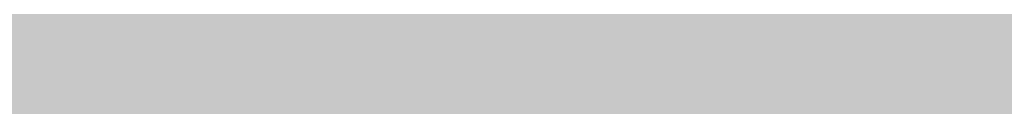
# Model space of a CAD drawing. Units: millimetres. Extents: x 0 to 2267, y 0 to 1823.
# Tile 53 of 256: x 1596.855 to 1600.369, y 1226.718 to 1227.02. Entities that reach past the tile are written whole.
import ezdxf

# ---------------------------------------------------------------- set-up
doc = ezdxf.new("R2010")
doc.units = ezdxf.units.MM
doc.header["$MEASUREMENT"] = 0
doc.layers.add('M-HATC', color=252, linetype='Continuous', lineweight=18)

msp = doc.modelspace()

# ---------------------------------------------------------------- hatches: boundary and pattern name
at = {"layer": 'M-HATC'}
h = msp.add_hatch(color=256, dxfattribs=at)
h.dxf.hatch_style = 1
h.paths.add_polyline_path([(2055.771, 1603.062), (1381.0868, 1603.062), (1381.0868, 1598.062), (2055.771, 1598.062)])
h.paths.add_polyline_path([(2055.771, 1598.062), (1381.0868, 1598.062), (1381.0868, 1593.062), (2055.771, 1593.062)])
h.paths.add_polyline_path([(2051.3074, 1536.7609), (1385.5504, 1536.7609), (1385.5504, 1526.7609), (1387.5504, 1526.7609), (1388.5366, 1525.0528), (1385.3319, 1521.2335), (1385.3319, 1521.2226), (2050.2542, 1522.7491), (2048.3212, 1525.0528), (2049.3074, 1526.7609), (2051.3074, 1526.7609)])
edge = h.paths.add_edge_path()
edge.add_arc((1847.5345, 1379.1492), 135, 222.603061, 222.890851, ccw=False)
edge.add_line((1748.1663, 1287.7656), (1683.0921, 1287.7656))
edge.add_arc((1583.7239, 1379.1492), 135, 317.109149, 317.396939, ccw=False)
edge.add_arc((1678.9686, 1290.6707), 5, 222.8909, 317.1091, ccw=False)
edge.add_arc((1774.2133, 1379.1492), 135, 222.603061, 222.890851, ccw=False)
edge.add_line((1674.8451, 1287.7656), (1609.7709, 1287.7656))
edge.add_arc((1510.4027, 1379.1492), 135, 317.109149, 317.396939, ccw=False)
edge.add_arc((1605.6474, 1290.6707), 5, 222.8909, 317.1091, ccw=False)
edge.add_arc((1700.8921, 1379.1492), 135, 222.603061, 222.890851, ccw=False)
edge.add_line((1601.5239, 1287.7656), (1536.4497, 1287.7656))
edge.add_arc((1437.0815, 1379.1492), 135, 317.109149, 317.396939, ccw=False)
edge.add_arc((1532.3262, 1290.6707), 5, 222.8909, 317.1091, ccw=False)
edge.add_arc((1627.5709, 1379.1492), 135, 222.603061, 222.890851, ccw=False)
edge.add_line((1528.2027, 1287.7656), (1505.9289, 1287.7656))
edge.add_spline(control_points=[(1505.9289, 1287.7656), (1504.2622, 1287.7656), (1504.2622, 1282.7656), (1505.9289, 1282.7656)], knot_values=[0, 0, 0, 0, 5, 5, 5, 5], degree=3, periodic=0)
edge.add_line((1505.9289, 1282.7656), (1930.9289, 1282.7656))
edge.add_spline(control_points=[(1930.9289, 1282.7656), (1932.5956, 1282.7656), (1932.5956, 1287.7656), (1930.9289, 1287.7656)], knot_values=[0, 0, 0, 0, 5, 5, 5, 5], degree=3, periodic=0)
edge.add_line((1930.9289, 1287.7656), (1903.0557, 1287.7656))
edge.add_arc((1803.6875, 1379.1492), 135, 317.109149, 317.396939, ccw=False)
edge.add_arc((1898.9322, 1290.6707), 5, 222.8909, 317.1091, ccw=False)
edge.add_arc((1994.1769, 1379.1492), 135, 222.603061, 222.890851, ccw=False)
edge.add_line((1894.8087, 1287.7656), (1829.7345, 1287.7656))
edge.add_arc((1730.3663, 1379.1492), 135, 317.109149, 317.396939, ccw=False)
edge.add_arc((1825.611, 1290.6707), 5, 222.8909, 317.1091, ccw=False)
edge.add_arc((1920.8557, 1379.1492), 135, 222.603061, 222.890851, ccw=False)
edge.add_line((1821.4875, 1287.7656), (1756.4133, 1287.7656))
edge.add_arc((1657.0451, 1379.1492), 135, 317.109149, 317.396939, ccw=False)
edge.add_arc((1752.2898, 1290.6707), 5, 222.8909, 317.1091, ccw=False)
edge = h.paths.add_edge_path()
edge.add_spline(control_points=[(1843.4289, 1227.2475), (1845.0956, 1227.2475), (1845.0956, 1232.2475), (1843.4289, 1232.2475)], knot_values=[0, 0, 0, 0, 5, 5, 5, 5], degree=3, periodic=0)
edge.add_line((1843.4289, 1232.2475), (1593.4289, 1232.2475))
edge.add_spline(control_points=[(1593.4289, 1232.2475), (1591.7622, 1232.2475), (1591.7622, 1227.2475), (1593.4289, 1227.2475)], knot_values=[0, 0, 0, 0, 5, 5, 5, 5], degree=3, periodic=0)
edge.add_line((1593.4289, 1227.2475), (1843.4289, 1227.2475))
h.paths.add_polyline_path([(1905.9289, 1127.4171), (1530.9289, 1127.4171, 0.414214), (1520.9289, 1117.4171), (1530.9289, 1117.4171), (1915.9289, 1117.4171, 0.414214)])
edge = h.paths.add_edge_path()
edge.add_arc((1397.0858, 1498.4078), 12.7299, 90.78215, 190.87871, ccw=False)
edge.add_line((1396.912, 1511.1365), (1428.0097, 1511.3488))
edge.add_line((1428.0097, 1511.3488), (1433.0097, 1511.3488))
edge.add_line((1433.0097, 1511.3488), (1434.439, 1511.3488))
edge.add_arc((1419.474, 1498.0804), 20, 41.561, 74.08211)
edge.add_line((1424.9592, 1517.3135), (1399.9351, 1517.2561))
edge.add_spline(control_points=[(1399.9307, 1517.2561), (1399.884, 1517.2131), (1399.8328, 1517.1689), (1399.7774, 1517.1236)], knot_values=[11.567499, 11.567499, 11.567499, 11.567499, 11.814249, 11.814249, 11.814249, 11.814249], degree=3, periodic=0)
edge.add_spline(control_points=[(1399.6328, 1517.0099), (1399.5831, 1516.9721), (1399.5307, 1516.9338), (1399.4759, 1516.8947)], knot_values=[11.167718, 11.167718, 11.167718, 11.167718, 11.365188, 11.365188, 11.365188, 11.365188], degree=3, periodic=0)
edge.add_spline(control_points=[(1399.3398, 1516.8001), (1399.1514, 1516.6719), (1398.9384, 1516.5377), (1398.704, 1516.3994)], knot_values=[10.376405, 10.376405, 10.376405, 10.376405, 11.00994, 11.00994, 11.00994, 11.00994], degree=3, periodic=0)
edge.add_spline(control_points=[(1398.6572, 1516.3719), (1398.5789, 1516.326), (1398.4983, 1516.2797), (1398.4155, 1516.2331)], knot_values=[10.125175, 10.125175, 10.125175, 10.125175, 10.334406, 10.334406, 10.334406, 10.334406], degree=3, periodic=0)
edge.add_spline(control_points=[(1398.2642, 1516.1487), (1398.196, 1516.1111), (1398.1263, 1516.0732), (1398.0555, 1516.0351)], knot_values=[9.832246, 9.832246, 9.832246, 9.832246, 9.999658, 9.999658, 9.999658, 9.999658], degree=3, periodic=0)
edge.add_spline(control_points=[(1397.9987, 1516.0048), (1397.7312, 1515.8621), (1397.446, 1515.7171), (1397.1466, 1515.5714)], knot_values=[9.161808, 9.161808, 9.161808, 9.161808, 9.787769, 9.787769, 9.787769, 9.787769], degree=3, periodic=0)
edge.add_spline(control_points=[(1397.1466, 1515.5714), (1396.8418, 1515.423), (1396.5222, 1515.274), (1396.1914, 1515.1262)], knot_values=[8.524455, 8.524455, 8.524455, 8.524455, 9.161808, 9.161808, 9.161808, 9.161808], degree=3, periodic=0)
edge.add_spline(control_points=[(1396.0777, 1515.0756), (1395.9854, 1515.0348), (1395.8922, 1514.994), (1395.7983, 1514.9534)], knot_values=[8.275193, 8.275193, 8.275193, 8.275193, 8.451726, 8.451726, 8.451726, 8.451726], degree=3, periodic=0)
edge.add_spline(control_points=[(1395.6018, 1514.8691), (1395.4997, 1514.8257), (1395.3968, 1514.7824), (1395.2932, 1514.7394)], knot_values=[7.962917, 7.962917, 7.962917, 7.962917, 8.152764, 8.152764, 8.152764, 8.152764], degree=3, periodic=0)
edge.add_spline(control_points=[(1395.2116, 1514.7057), (1394.8278, 1514.5475), (1394.4345, 1514.3929), (1394.0364, 1514.2442)], knot_values=[7.21254, 7.21254, 7.21254, 7.21254, 7.913148, 7.913148, 7.913148, 7.913148], degree=3, periodic=0)
edge.add_spline(control_points=[(1394.0364, 1514.2442), (1393.7076, 1514.1214), (1393.3754, 1514.0027), (1393.0427, 1513.8895)], knot_values=[6.633733, 6.633733, 6.633733, 6.633733, 7.21254, 7.21254, 7.21254, 7.21254], degree=3, periodic=0)
edge.add_spline(control_points=[(1392.8214, 1513.815), (1392.7198, 1513.7812), (1392.6181, 1513.7479), (1392.5166, 1513.7152)], knot_values=[6.328796, 6.328796, 6.328796, 6.328796, 6.505493, 6.505493, 6.505493, 6.505493], degree=3, periodic=0)
edge.add_spline(control_points=[(1392.5166, 1513.7152), (1392.3187, 1513.6515), (1392.1212, 1513.59), (1391.9244, 1513.531)], knot_values=[5.984605, 5.984605, 5.984605, 5.984605, 6.328796, 6.328796, 6.328796, 6.328796], degree=3, periodic=0)
edge.add_spline(control_points=[(1391.7915, 1513.4915), (1391.3122, 1513.3501), (1390.8384, 1513.2239), (1390.3784, 1513.1171)], knot_values=[5.066697, 5.066697, 5.066697, 5.066697, 5.907055, 5.907055, 5.907055, 5.907055], degree=3, periodic=0)
edge.add_spline(control_points=[(1390.3784, 1513.1171), (1390.1797, 1513.071), (1389.9836, 1513.0284), (1389.7907, 1512.9899)], knot_values=[4.70367, 4.70367, 4.70367, 4.70367, 5.066695, 5.066695, 5.066695, 5.066695], degree=3, periodic=0)
edge.add_spline(control_points=[(1389.422, 1512.9204), (1389.2459, 1512.8892), (1389.0729, 1512.8617), (1388.9036, 1512.8381)], knot_values=[4.130571, 4.130571, 4.130571, 4.130571, 4.469816, 4.469816, 4.469816, 4.469816], degree=3, periodic=0)
edge.add_spline(control_points=[(1388.9036, 1512.8381), (1388.591, 1512.7946), (1388.2911, 1512.7644), (1388.0071, 1512.7494)], knot_values=[3.504031, 3.504031, 3.504031, 3.504031, 4.130571, 4.130571, 4.130571, 4.130571], degree=3, periodic=0)
edge.add_spline(control_points=[(1387.9356, 1512.7459), (1387.8538, 1512.7423), (1387.7733, 1512.74), (1387.6944, 1512.739)], knot_values=[3.268866, 3.268866, 3.268866, 3.268866, 3.451164, 3.451164, 3.451164, 3.451164], degree=3, periodic=0)
edge.add_spline(control_points=[(1387.3351, 1512.7443), (1387.2076, 1512.7499), (1387.0847, 1512.7597), (1386.967, 1512.7739)], knot_values=[2.670686, 2.670686, 2.670686, 2.670686, 2.984, 2.984, 2.984, 2.984], degree=3, periodic=0)
edge.add_spline(control_points=[(1386.8327, 1512.7922), (1386.8209, 1512.7941), (1386.8092, 1512.7959), (1386.7975, 1512.7979)], knot_values=[2.516981, 2.516981, 2.516981, 2.516981, 2.549528, 2.549528, 2.549528, 2.549528], degree=3, periodic=0)
edge.add_spline(control_points=[(1386.4526, 1512.8735), (1386.4257, 1512.881), (1386.3993, 1512.889), (1386.3733, 1512.8972)], knot_values=[2.095869, 2.095869, 2.095869, 2.095869, 2.17941, 2.17941, 2.17941, 2.17941], degree=3, periodic=0)
edge.add_spline(control_points=[(1386.0691, 1513.0189), (1386.0634, 1513.0217), (1386.0577, 1513.0246), (1386.052, 1513.0275)], knot_values=[1.72453, 1.72453, 1.72453, 1.72453, 1.745933, 1.745933, 1.745933, 1.745933], degree=3, periodic=0)
edge.add_arc((1399.474, 1498.0804), 20, 131.82432, 180)
edge.add_arc((1630.3336, 1505.5484), 250.9708, 181.705176, 236.427975)
edge.add_arc((1605.3399, 1483.3044), 218.7822, 238.660829, 243.34961)
edge.add_arc((1647.0911, 1510.3592), 262.8986, 183.129836, 237.853442, ccw=False)
h.paths.add_polyline_path([(1406.5369, 1391.9644, 0.149382), (1491.5506, 1296.4418, -0.129517)], flags=17)
edge = h.paths.add_edge_path()
edge.add_arc((2037.3838, 1498.0804), 20, 0, 48.26587)
edge.add_spline(control_points=[(2050.6973, 1513.0052), (2050.6512, 1512.9847), (2050.6034, 1512.9655), (2050.5539, 1512.9477)], knot_values=[1.835652, 1.835652, 1.835652, 1.835652, 2.000781, 2.000781, 2.000781, 2.000781], degree=3, periodic=0)
edge.add_spline(control_points=[(2050.4616, 1512.9166), (2050.479, 1512.9221), (2050.4963, 1512.9277), (2050.5133, 1512.9335)], knot_values=[2.045477, 2.045477, 2.045477, 2.045477, 2.101389, 2.101389, 2.101389, 2.101389], degree=3, periodic=0)
edge.add_spline(control_points=[(2050.129, 1512.8342), (2050.1984, 1512.8473), (2050.2657, 1512.8623), (2050.3308, 1512.8792)], knot_values=[2.237629, 2.237629, 2.237629, 2.237629, 2.435841, 2.435841, 2.435841, 2.435841], degree=3, periodic=0)
edge.add_spline(control_points=[(2050.0946, 1512.8278), (2050.1061, 1512.8299), (2050.1176, 1512.832), (2050.129, 1512.8342)], knot_values=[2.435841, 2.435841, 2.435841, 2.435841, 2.468321, 2.468321, 2.468321, 2.468321], degree=3, periodic=0)
edge.add_spline(control_points=[(2049.7843, 1512.7851), (2049.8552, 1512.7922), (2049.9243, 1512.8008), (2049.9917, 1512.8109)], knot_values=[2.563852, 2.563852, 2.563852, 2.563852, 2.748541, 2.748541, 2.748541, 2.748541], degree=3, periodic=0)
edge.add_spline(control_points=[(2049.4052, 1512.7617), (2049.5364, 1512.7653), (2049.6629, 1512.773), (2049.7843, 1512.7851)], knot_values=[2.748541, 2.748541, 2.748541, 2.748541, 3.064882, 3.064882, 3.064882, 3.064882], degree=3, periodic=0)
edge.add_spline(control_points=[(2049.1698, 1512.7597), (2049.2336, 1512.7591), (2049.2965, 1512.7594), (2049.3584, 1512.7606)], knot_values=[3.102309, 3.102309, 3.102309, 3.102309, 3.2503, 3.2503, 3.2503, 3.2503], degree=3, periodic=0)
edge.add_spline(control_points=[(2048.8573, 1512.7691), (2048.9638, 1512.7638), (2049.068, 1512.7606), (2049.1698, 1512.7597)], knot_values=[3.2503, 3.2503, 3.2503, 3.2503, 3.486069, 3.486069, 3.486069, 3.486069], degree=3, periodic=0)
edge.add_spline(control_points=[(2048.6924, 1512.7789), (2048.3729, 1512.8009), (2048.0345, 1512.8411), (2047.6817, 1512.897)], knot_values=[3.606429, 3.606429, 3.606429, 3.606429, 4.2989, 4.2989, 4.2989, 4.2989], degree=3, periodic=0)
edge.add_spline(control_points=[(2047.6817, 1512.897), (2047.5458, 1512.9185), (2047.4077, 1512.9424), (2047.2678, 1512.9685)], knot_values=[4.2989, 4.2989, 4.2989, 4.2989, 4.565769, 4.565769, 4.565769, 4.565769], degree=3, periodic=0)
edge.add_spline(control_points=[(2047.2678, 1512.9685), (2047.1449, 1512.9914), (2047.0207, 1513.016), (2046.8951, 1513.0422)], knot_values=[4.565769, 4.565769, 4.565769, 4.565769, 4.799971, 4.799971, 4.799971, 4.799971], degree=3, periodic=0)
edge.add_spline(control_points=[(2046.8951, 1513.0422), (2046.5286, 1513.1188), (2046.1513, 1513.209), (2045.7676, 1513.3107)], knot_values=[4.799971, 4.799971, 4.799971, 4.799971, 5.483718, 5.483718, 5.483718, 5.483718], degree=3, periodic=0)
edge.add_spline(control_points=[(2045.7676, 1513.3107), (2045.3724, 1513.4154), (2044.9704, 1513.5322), (2044.5662, 1513.6588)], knot_values=[5.483718, 5.483718, 5.483718, 5.483718, 6.187866, 6.187866, 6.187866, 6.187866], degree=3, periodic=0)
edge.add_spline(control_points=[(2044.5662, 1513.6588), (2044.4149, 1513.7061), (2044.2633, 1513.7549), (2044.1116, 1513.8048)], knot_values=[6.187866, 6.187866, 6.187866, 6.187866, 6.451551, 6.451551, 6.451551, 6.451551], degree=3, periodic=0)
edge.add_spline(control_points=[(2044.1116, 1513.8048), (2043.9967, 1513.8427), (2043.8817, 1513.8813), (2043.7668, 1513.9205)], knot_values=[6.451551, 6.451551, 6.451551, 6.451551, 6.651434, 6.651434, 6.651434, 6.651434], degree=3, periodic=0)
edge.add_spline(control_points=[(2043.7668, 1513.9205), (2043.3716, 1514.0554), (2042.9774, 1514.1979), (2042.5886, 1514.3458)], knot_values=[6.651434, 6.651434, 6.651434, 6.651434, 7.338879, 7.338879, 7.338879, 7.338879], degree=3, periodic=0)
edge.add_spline(control_points=[(2042.5886, 1514.3458), (2042.1643, 1514.5071), (2041.7465, 1514.6749), (2041.3409, 1514.846)], knot_values=[7.338879, 7.338879, 7.338879, 7.338879, 8.089209, 8.089209, 8.089209, 8.089209], degree=3, periodic=0)
edge.add_spline(control_points=[(2041.3409, 1514.846), (2041.1028, 1514.9465), (2040.869, 1515.0481), (2040.6405, 1515.1502)], knot_values=[8.089209, 8.089209, 8.089209, 8.089209, 8.529587, 8.529587, 8.529587, 8.529587], degree=3, periodic=0)
edge.add_spline(control_points=[(2040.51, 1515.2089), (2040.0824, 1515.4022), (2039.6747, 1515.5971), (2039.295, 1515.7894)], knot_values=[8.613818, 8.613818, 8.613818, 8.613818, 9.44571, 9.44571, 9.44571, 9.44571], degree=3, periodic=0)
edge.add_spline(control_points=[(2039.295, 1515.7894), (2039.0618, 1515.9075), (2038.8391, 1516.0246), (2038.6288, 1516.1398)], knot_values=[9.44571, 9.44571, 9.44571, 9.44571, 9.956404, 9.956404, 9.956404, 9.956404], degree=3, periodic=0)
edge.add_spline(control_points=[(2038.6288, 1516.1398), (2038.5187, 1516.2001), (2038.4121, 1516.2598), (2038.309, 1516.3189)], knot_values=[9.956404, 9.956404, 9.956404, 9.956404, 10.223542, 10.223542, 10.223542, 10.223542], degree=3, periodic=0)
edge.add_spline(control_points=[(2038.309, 1516.3189), (2038.2138, 1516.3735), (2038.1216, 1516.4276), (2038.0328, 1516.481)], knot_values=[10.223542, 10.223542, 10.223542, 10.223542, 10.47051, 10.47051, 10.47051, 10.47051], degree=3, periodic=0)
edge.add_spline(control_points=[(2038.0328, 1516.481), (2037.7855, 1516.6296), (2037.5639, 1516.773), (2037.3722, 1516.909)], knot_values=[10.47051, 10.47051, 10.47051, 10.47051, 11.15767, 11.15767, 11.15767, 11.15767], degree=3, periodic=0)
edge.add_spline(control_points=[(2037.3722, 1516.909), (2037.2789, 1516.9752), (2037.1927, 1517.0396), (2037.1142, 1517.102)], knot_values=[11.15767, 11.15767, 11.15767, 11.15767, 11.49227, 11.49227, 11.49227, 11.49227], degree=3, periodic=0)
edge.add_spline(control_points=[(2036.8564, 1517.3259), (2036.9148, 1517.2692), (2036.9814, 1517.2103), (2037.0557, 1517.1492)], knot_values=[11.577341, 11.577341, 11.577341, 11.577341, 11.91035, 11.91035, 11.91035, 11.91035], degree=3, periodic=0)
edge.add_spline(control_points=[(2036.8074, 1517.3748), (2036.823, 1517.3587), (2036.8393, 1517.3424), (2036.8564, 1517.3259)], knot_values=[11.91035, 11.91035, 11.91035, 11.91035, 12.007402, 12.007402, 12.007402, 12.007402], degree=3, periodic=0)
edge.add_spline(control_points=[(2036.7017, 1517.494), (2036.7104, 1517.483), (2036.7196, 1517.4719), (2036.7291, 1517.4606)], knot_values=[12.184155, 12.184155, 12.184155, 12.184155, 12.255409, 12.255409, 12.255409, 12.255409], degree=3, periodic=0)
edge.add_spline(control_points=[(2036.6159, 1517.6205), (2036.62, 1517.613), (2036.6243, 1517.6055), (2036.6289, 1517.5979)], knot_values=[12.487913, 12.487913, 12.487913, 12.487913, 12.541035, 12.541035, 12.541035, 12.541035], degree=3, periodic=0)
edge.add_spline(control_points=[(2036.5635, 1517.786), (2036.5637, 1517.7794), (2036.5642, 1517.7726), (2036.565, 1517.7658)], knot_values=[12.911761, 12.911761, 12.911761, 12.911761, 12.968286, 12.968286, 12.968286, 12.968286], degree=3, periodic=0)
edge.add_spline(control_points=[(2036.6166, 1517.9304), (2036.6125, 1517.9259), (2036.6086, 1517.9212), (2036.6049, 1517.9165)], knot_values=[13.382527, 13.382527, 13.382527, 13.382527, 13.433791, 13.433791, 13.433791, 13.433791], degree=3, periodic=0)
edge.add_spline(control_points=[(2036.749, 1518.017), (2036.7361, 1518.0116), (2036.7239, 1518.006), (2036.7124, 1518.0002)], knot_values=[13.726299, 13.726299, 13.726299, 13.726299, 13.809928, 13.809928, 13.809928, 13.809928], degree=3, periodic=0)
edge.add_spline(control_points=[(2036.8604, 1518.0528), (2036.8386, 1518.0474), (2036.8181, 1518.0416), (2036.7988, 1518.0353)], knot_values=[13.910887, 13.910887, 13.910887, 13.910887, 14.02153, 14.02153, 14.02153, 14.02153], degree=3, periodic=0)
edge.add_line((2036.9639, 1518.0804), (2032.3838, 1518.0804))
edge.add_line((2032.3838, 1518.0804), (2027.3838, 1518.0804))
edge.add_line((2027.3838, 1518.0804), (2022.3838, 1518.0804))
edge.add_line((2022.3838, 1518.0804), (2017.3838, 1518.0804))
edge.add_arc((2017.3838, 1498.0804), 20, 90, 138.439)
edge.add_line((2002.4188, 1511.3488), (2003.8481, 1511.3488))
edge.add_line((2003.8481, 1511.3488), (2008.8481, 1511.3488))
edge.add_line((2008.8481, 1511.3488), (2039.772, 1511.1377))
edge.add_arc((2039.772, 1498.4078), 12.7299, -10.87871, 90, ccw=False)
edge.add_arc((1789.7668, 1510.3592), 262.8986, 302.146558, 356.870164, ccw=False)
edge.add_arc((1831.5179, 1483.3044), 218.7822, 296.65039, 301.339171)
edge.add_arc((1806.5242, 1505.5484), 250.9708, 303.572025, 358.294824)
h.paths.add_polyline_path([(2030.321, 1391.9644, -0.129517), (1945.3072, 1296.4418, 0.149382)], flags=17)
edge = h.paths.add_edge_path()
edge.add_spline(control_points=[(2037.2464, 1518.0821), (2037.2898, 1518.081), (2037.3355, 1518.0804), (2037.3838, 1518.0804)], knot_values=[0.000012, 0.000012, 0.000012, 0.000012, 0.144754, 0.144754, 0.144754, 0.144754], degree=3, periodic=0)
edge.add_line((2037.3357, 1518.0804), (2037.0096, 1518.0804))
edge.add_spline(control_points=[(2037.0096, 1518.0804), (2036.9822, 1518.0768), (2036.956, 1518.0727), (2036.9312, 1518.0681)], knot_values=[14.13465, 14.13465, 14.13465, 14.13465, 14.247197, 14.247197, 14.247197, 14.247197], degree=3, periodic=0)
edge.add_spline(control_points=[(2036.9312, 1518.0681), (2036.9276, 1518.0674), (2036.9241, 1518.0667), (2036.9205, 1518.0661)], knot_values=[14.118315, 14.118315, 14.118315, 14.118315, 14.13465, 14.13465, 14.13465, 14.13465], degree=3, periodic=0)
edge.add_spline(control_points=[(2036.9205, 1518.0661), (2036.9118, 1518.0644), (2036.9032, 1518.0626), (2036.8948, 1518.0608)], knot_values=[14.078086, 14.078086, 14.078086, 14.078086, 14.118315, 14.118315, 14.118315, 14.118315], degree=3, periodic=0)
edge.add_spline(control_points=[(2036.8948, 1518.0608), (2036.883, 1518.0583), (2036.8716, 1518.0556), (2036.8604, 1518.0528)], knot_values=[14.02153, 14.02153, 14.02153, 14.02153, 14.078086, 14.078086, 14.078086, 14.078086], degree=3, periodic=0)
edge.add_spline(control_points=[(2036.8604, 1518.0528), (2036.8386, 1518.0474), (2036.8181, 1518.0416), (2036.7988, 1518.0353)], knot_values=[13.910887, 13.910887, 13.910887, 13.910887, 14.02153, 14.02153, 14.02153, 14.02153], degree=3, periodic=0)
edge.add_spline(control_points=[(2036.7988, 1518.0353), (2036.7981, 1518.035), (2036.7974, 1518.0348), (2036.7967, 1518.0346)], knot_values=[13.906906, 13.906906, 13.906906, 13.906906, 13.910887, 13.910887, 13.910887, 13.910887], degree=3, periodic=0)
edge.add_spline(control_points=[(2036.7967, 1518.0346), (2036.7882, 1518.0318), (2036.7799, 1518.0289), (2036.7719, 1518.0259)], knot_values=[13.857826, 13.857826, 13.857826, 13.857826, 13.906906, 13.906906, 13.906906, 13.906906], degree=3, periodic=0)
edge.add_spline(control_points=[(2036.7719, 1518.0259), (2036.764, 1518.023), (2036.7564, 1518.02), (2036.749, 1518.017)], knot_values=[13.809928, 13.809928, 13.809928, 13.809928, 13.857826, 13.857826, 13.857826, 13.857826], degree=3, periodic=0)
edge.add_spline(control_points=[(2036.749, 1518.017), (2036.7361, 1518.0116), (2036.7239, 1518.006), (2036.7124, 1518.0002)], knot_values=[13.726299, 13.726299, 13.726299, 13.726299, 13.809928, 13.809928, 13.809928, 13.809928], degree=3, periodic=0)
edge.add_spline(control_points=[(2036.7124, 1518.0002), (2036.7121, 1518), (2036.7118, 1517.9999), (2036.7115, 1517.9997)], knot_values=[13.723993, 13.723993, 13.723993, 13.723993, 13.726299, 13.726299, 13.726299, 13.726299], degree=3, periodic=0)
edge.add_spline(control_points=[(2036.7115, 1517.9997), (2036.7063, 1517.9971), (2036.7013, 1517.9944), (2036.6965, 1517.9917)], knot_values=[13.686536, 13.686536, 13.686536, 13.686536, 13.723993, 13.723993, 13.723993, 13.723993], degree=3, periodic=0)
edge.add_spline(control_points=[(2036.6965, 1517.9917), (2036.6919, 1517.9891), (2036.6874, 1517.9865), (2036.6831, 1517.9839)], knot_values=[13.651251, 13.651251, 13.651251, 13.651251, 13.686536, 13.686536, 13.686536, 13.686536], degree=3, periodic=0)
edge.add_spline(control_points=[(2036.6831, 1517.9839), (2036.6764, 1517.9798), (2036.67, 1517.9757), (2036.6639, 1517.9714)], knot_values=[13.596804, 13.596804, 13.596804, 13.596804, 13.651251, 13.651251, 13.651251, 13.651251], degree=3, periodic=0)
edge.add_spline(control_points=[(2036.6639, 1517.9714), (2036.6636, 1517.9712), (2036.6633, 1517.9709), (2036.6629, 1517.9707)], knot_values=[13.593956, 13.593956, 13.593956, 13.593956, 13.596804, 13.596804, 13.596804, 13.596804], degree=3, periodic=0)
edge.add_spline(control_points=[(2036.6629, 1517.9707), (2036.6603, 1517.9689), (2036.6577, 1517.967), (2036.6552, 1517.9651)], knot_values=[13.570322, 13.570322, 13.570322, 13.570322, 13.593956, 13.593956, 13.593956, 13.593956], degree=3, periodic=0)
edge.add_spline(control_points=[(2036.6552, 1517.9651), (2036.6525, 1517.9631), (2036.6499, 1517.9611), (2036.6474, 1517.9591)], knot_values=[13.545477, 13.545477, 13.545477, 13.545477, 13.570322, 13.570322, 13.570322, 13.570322], degree=3, periodic=0)
edge.add_spline(control_points=[(2036.6474, 1517.9591), (2036.6472, 1517.9589), (2036.6471, 1517.9588), (2036.6469, 1517.9587)], knot_values=[13.543931, 13.543931, 13.543931, 13.543931, 13.545477, 13.545477, 13.545477, 13.545477], degree=3, periodic=0)
edge.add_spline(control_points=[(2036.6469, 1517.9587), (2036.6412, 1517.9541), (2036.6358, 1517.9494), (2036.6307, 1517.9447)], knot_values=[13.488237, 13.488237, 13.488237, 13.488237, 13.543931, 13.543931, 13.543931, 13.543931], degree=3, periodic=0)
edge.add_spline(control_points=[(2036.6307, 1517.9447), (2036.6282, 1517.9423), (2036.6257, 1517.9399), (2036.6233, 1517.9374)], knot_values=[13.460307, 13.460307, 13.460307, 13.460307, 13.488237, 13.488237, 13.488237, 13.488237], degree=3, periodic=0)
edge.add_spline(control_points=[(2036.6233, 1517.9374), (2036.6215, 1517.9356), (2036.6198, 1517.9338), (2036.6181, 1517.932)], knot_values=[13.439712, 13.439712, 13.439712, 13.439712, 13.460307, 13.460307, 13.460307, 13.460307], degree=3, periodic=0)
edge.add_spline(control_points=[(2036.6181, 1517.932), (2036.6176, 1517.9315), (2036.6171, 1517.9309), (2036.6166, 1517.9304)], knot_values=[13.433791, 13.433791, 13.433791, 13.433791, 13.439712, 13.439712, 13.439712, 13.439712], degree=3, periodic=0)
edge.add_spline(control_points=[(2036.6166, 1517.9304), (2036.6125, 1517.9259), (2036.6086, 1517.9212), (2036.6049, 1517.9165)], knot_values=[13.382527, 13.382527, 13.382527, 13.382527, 13.433791, 13.433791, 13.433791, 13.433791], degree=3, periodic=0)
edge.add_spline(control_points=[(2036.6049, 1517.9165), (2036.6026, 1517.9135), (2036.6004, 1517.9104), (2036.5982, 1517.9074)], knot_values=[13.350017, 13.350017, 13.350017, 13.350017, 13.382527, 13.382527, 13.382527, 13.382527], degree=3, periodic=0)
edge.add_spline(control_points=[(2036.5982, 1517.9074), (2036.5972, 1517.9059), (2036.5962, 1517.9043), (2036.5952, 1517.9028)], knot_values=[13.333922, 13.333922, 13.333922, 13.333922, 13.350017, 13.350017, 13.350017, 13.350017], degree=3, periodic=0)
edge.add_spline(control_points=[(2036.5952, 1517.9028), (2036.5945, 1517.9018), (2036.5939, 1517.9009), (2036.5933, 1517.8999)], knot_values=[13.323828, 13.323828, 13.323828, 13.323828, 13.333922, 13.333922, 13.333922, 13.333922], degree=3, periodic=0)
edge.add_spline(control_points=[(2036.5933, 1517.8999), (2036.5905, 1517.8955), (2036.5879, 1517.8909), (2036.5855, 1517.8864)], knot_values=[13.277545, 13.277545, 13.277545, 13.277545, 13.323828, 13.323828, 13.323828, 13.323828], degree=3, periodic=0)
edge.add_spline(control_points=[(2036.5855, 1517.8864), (2036.5836, 1517.8827), (2036.5817, 1517.8789), (2036.5801, 1517.8751)], knot_values=[13.240119, 13.240119, 13.240119, 13.240119, 13.277545, 13.277545, 13.277545, 13.277545], degree=3, periodic=0)
edge.add_spline(control_points=[(2036.5801, 1517.8751), (2036.5795, 1517.8739), (2036.579, 1517.8727), (2036.5785, 1517.8715)], knot_values=[13.228211, 13.228211, 13.228211, 13.228211, 13.240119, 13.240119, 13.240119, 13.240119], degree=3, periodic=0)
edge.add_spline(control_points=[(2036.5785, 1517.8715), (2036.578, 1517.8702), (2036.5774, 1517.869), (2036.5769, 1517.8677)], knot_values=[13.215717, 13.215717, 13.215717, 13.215717, 13.228211, 13.228211, 13.228211, 13.228211], degree=3, periodic=0)
edge.add_spline(control_points=[(2036.5769, 1517.8677), (2036.5755, 1517.864), (2036.5741, 1517.8603), (2036.5729, 1517.8565)], knot_values=[13.179847, 13.179847, 13.179847, 13.179847, 13.215717, 13.215717, 13.215717, 13.215717], degree=3, periodic=0)
edge.add_spline(control_points=[(2036.5729, 1517.8565), (2036.5713, 1517.8515), (2036.5699, 1517.8464), (2036.5687, 1517.8413)], knot_values=[13.132017, 13.132017, 13.132017, 13.132017, 13.179847, 13.179847, 13.179847, 13.179847], degree=3, periodic=0)
edge.add_spline(control_points=[(2036.5687, 1517.8413), (2036.5684, 1517.8402), (2036.5682, 1517.8392), (2036.568, 1517.8382)], knot_values=[13.122482, 13.122482, 13.122482, 13.122482, 13.132017, 13.132017, 13.132017, 13.132017], degree=3, periodic=0)
edge.add_spline(control_points=[(2036.568, 1517.8382), (2036.5676, 1517.8363), (2036.5672, 1517.8345), (2036.5669, 1517.8327)], knot_values=[13.105592, 13.105592, 13.105592, 13.105592, 13.122482, 13.122482, 13.122482, 13.122482], degree=3, periodic=0)
edge.add_spline(control_points=[(2036.5669, 1517.8327), (2036.5662, 1517.8292), (2036.5657, 1517.8257), (2036.5652, 1517.8222)], knot_values=[13.074063, 13.074063, 13.074063, 13.074063, 13.105592, 13.105592, 13.105592, 13.105592], degree=3, periodic=0)
edge.add_spline(control_points=[(2036.5652, 1517.8222), (2036.5652, 1517.8222), (2036.5652, 1517.8222), (2036.5652, 1517.8222)], knot_values=[13.074043, 13.074043, 13.074043, 13.074043, 13.074063, 13.074063, 13.074063, 13.074063], degree=3, periodic=0)
edge.add_spline(control_points=[(2036.5652, 1517.8222), (2036.5644, 1517.8164), (2036.5639, 1517.8106), (2036.5636, 1517.8046)], knot_values=[13.021884, 13.021884, 13.021884, 13.021884, 13.074043, 13.074043, 13.074043, 13.074043], degree=3, periodic=0)
edge.add_spline(control_points=[(2036.5636, 1517.8046), (2036.5636, 1517.804), (2036.5636, 1517.8034), (2036.5635, 1517.8028)], knot_values=[13.01674, 13.01674, 13.01674, 13.01674, 13.021884, 13.021884, 13.021884, 13.021884], degree=3, periodic=0)
edge.add_spline(control_points=[(2036.5635, 1517.8028), (2036.5634, 1517.8005), (2036.5634, 1517.7982), (2036.5634, 1517.7958)], knot_values=[12.996438, 12.996438, 12.996438, 12.996438, 13.01674, 13.01674, 13.01674, 13.01674], degree=3, periodic=0)
edge.add_spline(control_points=[(2036.5634, 1517.7958), (2036.5633, 1517.7926), (2036.5634, 1517.7893), (2036.5635, 1517.786)], knot_values=[12.968286, 12.968286, 12.968286, 12.968286, 12.996438, 12.996438, 12.996438, 12.996438], degree=3, periodic=0)
edge.add_spline(control_points=[(2036.5635, 1517.786), (2036.5637, 1517.7794), (2036.5642, 1517.7726), (2036.565, 1517.7658)], knot_values=[12.911761, 12.911761, 12.911761, 12.911761, 12.968286, 12.968286, 12.968286, 12.968286], degree=3, periodic=0)
edge.add_spline(control_points=[(2036.565, 1517.7658), (2036.565, 1517.7657), (2036.565, 1517.7656), (2036.565, 1517.7656)], knot_values=[12.911017, 12.911017, 12.911017, 12.911017, 12.911761, 12.911761, 12.911761, 12.911761], degree=3, periodic=0)
edge.add_spline(control_points=[(2036.565, 1517.7656), (2036.5654, 1517.7625), (2036.5658, 1517.7593), (2036.5663, 1517.7562)], knot_values=[12.88528, 12.88528, 12.88528, 12.88528, 12.911017, 12.911017, 12.911017, 12.911017], degree=3, periodic=0)
edge.add_spline(control_points=[(2036.5663, 1517.7562), (2036.5667, 1517.7534), (2036.5672, 1517.7506), (2036.5677, 1517.7478)], knot_values=[12.862519, 12.862519, 12.862519, 12.862519, 12.88528, 12.88528, 12.88528, 12.88528], degree=3, periodic=0)
edge.add_spline(control_points=[(2036.5677, 1517.7478), (2036.5678, 1517.7474), (2036.5679, 1517.7469), (2036.568, 1517.7465)], knot_values=[12.858885, 12.858885, 12.858885, 12.858885, 12.862519, 12.862519, 12.862519, 12.862519], degree=3, periodic=0)
edge.add_spline(control_points=[(2036.568, 1517.7465), (2036.5692, 1517.7399), (2036.5707, 1517.7332), (2036.5724, 1517.7264)], knot_values=[12.8053, 12.8053, 12.8053, 12.8053, 12.858885, 12.858885, 12.858885, 12.858885], degree=3, periodic=0)
edge.add_spline(control_points=[(2036.5724, 1517.7264), (2036.5734, 1517.7226), (2036.5745, 1517.7187), (2036.5756, 1517.7149)], knot_values=[12.775176, 12.775176, 12.775176, 12.775176, 12.8053, 12.8053, 12.8053, 12.8053], degree=3, periodic=0)
edge.add_spline(control_points=[(2036.5756, 1517.7149), (2036.5763, 1517.7125), (2036.577, 1517.7102), (2036.5778, 1517.7078)], knot_values=[12.756759, 12.756759, 12.756759, 12.756759, 12.775176, 12.775176, 12.775176, 12.775176], degree=3, periodic=0)
edge.add_spline(control_points=[(2036.5778, 1517.7078), (2036.5781, 1517.7067), (2036.5784, 1517.7057), (2036.5787, 1517.7047)], knot_values=[12.748742, 12.748742, 12.748742, 12.748742, 12.756759, 12.756759, 12.756759, 12.756759], degree=3, periodic=0)
edge.add_spline(control_points=[(2036.5787, 1517.7047), (2036.5808, 1517.6983), (2036.5831, 1517.6919), (2036.5856, 1517.6854)], knot_values=[12.69959, 12.69959, 12.69959, 12.69959, 12.748742, 12.748742, 12.748742, 12.748742], degree=3, periodic=0)
edge.add_spline(control_points=[(2036.5856, 1517.6854), (2036.5876, 1517.68), (2036.5898, 1517.6746), (2036.5921, 1517.6692)], knot_values=[12.659038, 12.659038, 12.659038, 12.659038, 12.69959, 12.69959, 12.69959, 12.69959], degree=3, periodic=0)
edge.add_spline(control_points=[(2036.5921, 1517.6692), (2036.594, 1517.6648), (2036.5959, 1517.6605), (2036.5979, 1517.6561)], knot_values=[12.626806, 12.626806, 12.626806, 12.626806, 12.659038, 12.659038, 12.659038, 12.659038], degree=3, periodic=0)
edge.add_spline(control_points=[(2036.5979, 1517.6561), (2036.5984, 1517.6551), (2036.5989, 1517.6541), (2036.5993, 1517.6531)], knot_values=[12.619394, 12.619394, 12.619394, 12.619394, 12.626806, 12.626806, 12.626806, 12.626806], degree=3, periodic=0)
edge.add_spline(control_points=[(2036.5993, 1517.6531), (2036.6043, 1517.6424), (2036.6099, 1517.6315), (2036.6159, 1517.6205)], knot_values=[12.541039, 12.541039, 12.541039, 12.541039, 12.619394, 12.619394, 12.619394, 12.619394], degree=3, periodic=0)
edge.add_spline(control_points=[(2036.6159, 1517.6205), (2036.6159, 1517.6205), (2036.6159, 1517.6205), (2036.6159, 1517.6205)], knot_values=[12.541035, 12.541035, 12.541035, 12.541035, 12.541039, 12.541039, 12.541039, 12.541039], degree=3, periodic=0)
edge.add_spline(control_points=[(2036.6159, 1517.6205), (2036.62, 1517.613), (2036.6243, 1517.6055), (2036.6289, 1517.5979)], knot_values=[12.487913, 12.487913, 12.487913, 12.487913, 12.541035, 12.541035, 12.541035, 12.541035], degree=3, periodic=0)
edge.add_spline(control_points=[(2036.6289, 1517.5979), (2036.6326, 1517.5916), (2036.6365, 1517.5853), (2036.6406, 1517.5789)], knot_values=[12.443982, 12.443982, 12.443982, 12.443982, 12.487913, 12.487913, 12.487913, 12.487913], degree=3, periodic=0)
edge.add_spline(control_points=[(2036.6406, 1517.5789), (2036.6414, 1517.5776), (2036.6423, 1517.5763), (2036.6431, 1517.5749)], knot_values=[12.434996, 12.434996, 12.434996, 12.434996, 12.443982, 12.443982, 12.443982, 12.443982], degree=3, periodic=0)
edge.add_spline(control_points=[(2036.6431, 1517.5749), (2036.6531, 1517.5596), (2036.6639, 1517.5439), (2036.6756, 1517.528)], knot_values=[12.329647, 12.329647, 12.329647, 12.329647, 12.434996, 12.434996, 12.434996, 12.434996], degree=3, periodic=0)
edge.add_spline(control_points=[(2036.6756, 1517.528), (2036.6839, 1517.5168), (2036.6925, 1517.5055), (2036.7017, 1517.494)], knot_values=[12.255409, 12.255409, 12.255409, 12.255409, 12.329647, 12.329647, 12.329647, 12.329647], degree=3, periodic=0)
edge.add_spline(control_points=[(2036.7017, 1517.494), (2036.7104, 1517.483), (2036.7196, 1517.4719), (2036.7291, 1517.4606)], knot_values=[12.184155, 12.184155, 12.184155, 12.184155, 12.255409, 12.255409, 12.255409, 12.255409], degree=3, periodic=0)
edge.add_spline(control_points=[(2036.7291, 1517.4606), (2036.7436, 1517.4435), (2036.759, 1517.4262), (2036.7753, 1517.4085)], knot_values=[12.075961, 12.075961, 12.075961, 12.075961, 12.184155, 12.184155, 12.184155, 12.184155], degree=3, periodic=0)
edge.add_spline(control_points=[(2036.7753, 1517.4085), (2036.7763, 1517.4075), (2036.7773, 1517.4064), (2036.7783, 1517.4054)], knot_values=[12.069502, 12.069502, 12.069502, 12.069502, 12.075961, 12.075961, 12.075961, 12.075961], degree=3, periodic=0)
edge.add_spline(control_points=[(2036.7783, 1517.4054), (2036.7877, 1517.3953), (2036.7974, 1517.385), (2036.8074, 1517.3748)], knot_values=[12.007402, 12.007402, 12.007402, 12.007402, 12.069502, 12.069502, 12.069502, 12.069502], degree=3, periodic=0)
edge.add_spline(control_points=[(2036.8074, 1517.3748), (2036.823, 1517.3587), (2036.8393, 1517.3424), (2036.8564, 1517.3259)], knot_values=[11.91035, 11.91035, 11.91035, 11.91035, 12.007402, 12.007402, 12.007402, 12.007402], degree=3, periodic=0)
edge.add_spline(control_points=[(2036.8564, 1517.3259), (2036.9148, 1517.2692), (2036.9814, 1517.2103), (2037.0557, 1517.1492)], knot_values=[11.577341, 11.577341, 11.577341, 11.577341, 11.91035, 11.91035, 11.91035, 11.91035], degree=3, periodic=0)
edge.add_spline(control_points=[(2037.0557, 1517.1492), (2037.0747, 1517.1336), (2037.0942, 1517.1179), (2037.1142, 1517.102)], knot_values=[11.49227, 11.49227, 11.49227, 11.49227, 11.577341, 11.577341, 11.577341, 11.577341], degree=3, periodic=0)
edge.add_spline(control_points=[(2037.1142, 1517.102), (2037.1927, 1517.0396), (2037.2789, 1516.9752), (2037.3722, 1516.909)], knot_values=[11.15767, 11.15767, 11.15767, 11.15767, 11.49227, 11.49227, 11.49227, 11.49227], degree=3, periodic=0)
edge.add_spline(control_points=[(2037.3722, 1516.909), (2037.5639, 1516.773), (2037.7855, 1516.6296), (2038.0328, 1516.481)], knot_values=[10.47051, 10.47051, 10.47051, 10.47051, 11.15767, 11.15767, 11.15767, 11.15767], degree=3, periodic=0)
edge.add_spline(control_points=[(2038.0328, 1516.481), (2038.1216, 1516.4276), (2038.2138, 1516.3735), (2038.309, 1516.3189)], knot_values=[10.223542, 10.223542, 10.223542, 10.223542, 10.47051, 10.47051, 10.47051, 10.47051], degree=3, periodic=0)
edge.add_spline(control_points=[(2038.309, 1516.3189), (2038.4121, 1516.2598), (2038.5187, 1516.2001), (2038.6288, 1516.1398)], knot_values=[9.956404, 9.956404, 9.956404, 9.956404, 10.223542, 10.223542, 10.223542, 10.223542], degree=3, periodic=0)
edge.add_spline(control_points=[(2038.6288, 1516.1398), (2038.8391, 1516.0246), (2039.0618, 1515.9075), (2039.295, 1515.7894)], knot_values=[9.44571, 9.44571, 9.44571, 9.44571, 9.956404, 9.956404, 9.956404, 9.956404], degree=3, periodic=0)
edge.add_spline(control_points=[(2039.295, 1515.7894), (2039.6747, 1515.5971), (2040.0824, 1515.4022), (2040.51, 1515.2089)], knot_values=[8.613818, 8.613818, 8.613818, 8.613818, 9.44571, 9.44571, 9.44571, 9.44571], degree=3, periodic=0)
edge.add_spline(control_points=[(2040.51, 1515.2089), (2040.5533, 1515.1893), (2040.5968, 1515.1697), (2040.6405, 1515.1502)], knot_values=[8.529587, 8.529587, 8.529587, 8.529587, 8.613818, 8.613818, 8.613818, 8.613818], degree=3, periodic=0)
edge.add_spline(control_points=[(2040.6405, 1515.1502), (2040.869, 1515.0481), (2041.1028, 1514.9465), (2041.3409, 1514.846)], knot_values=[8.089209, 8.089209, 8.089209, 8.089209, 8.529587, 8.529587, 8.529587, 8.529587], degree=3, periodic=0)
edge.add_spline(control_points=[(2041.3409, 1514.846), (2041.7465, 1514.6749), (2042.1643, 1514.5071), (2042.5886, 1514.3458)], knot_values=[7.338879, 7.338879, 7.338879, 7.338879, 8.089209, 8.089209, 8.089209, 8.089209], degree=3, periodic=0)
edge.add_spline(control_points=[(2042.5886, 1514.3458), (2042.9774, 1514.1979), (2043.3716, 1514.0554), (2043.7668, 1513.9205)], knot_values=[6.651434, 6.651434, 6.651434, 6.651434, 7.338879, 7.338879, 7.338879, 7.338879], degree=3, periodic=0)
edge.add_spline(control_points=[(2043.7668, 1513.9205), (2043.8817, 1513.8813), (2043.9967, 1513.8427), (2044.1116, 1513.8048)], knot_values=[6.451551, 6.451551, 6.451551, 6.451551, 6.651434, 6.651434, 6.651434, 6.651434], degree=3, periodic=0)
edge.add_spline(control_points=[(2044.1116, 1513.8048), (2044.2633, 1513.7549), (2044.4149, 1513.7061), (2044.5662, 1513.6588)], knot_values=[6.187866, 6.187866, 6.187866, 6.187866, 6.451551, 6.451551, 6.451551, 6.451551], degree=3, periodic=0)
edge.add_spline(control_points=[(2044.5662, 1513.6588), (2044.9704, 1513.5322), (2045.3724, 1513.4154), (2045.7676, 1513.3107)], knot_values=[5.483718, 5.483718, 5.483718, 5.483718, 6.187866, 6.187866, 6.187866, 6.187866], degree=3, periodic=0)
edge.add_spline(control_points=[(2045.7676, 1513.3107), (2046.1513, 1513.209), (2046.5286, 1513.1188), (2046.8951, 1513.0422)], knot_values=[4.799971, 4.799971, 4.799971, 4.799971, 5.483718, 5.483718, 5.483718, 5.483718], degree=3, periodic=0)
edge.add_spline(control_points=[(2046.8951, 1513.0422), (2047.0207, 1513.016), (2047.1449, 1512.9914), (2047.2678, 1512.9685)], knot_values=[4.565769, 4.565769, 4.565769, 4.565769, 4.799971, 4.799971, 4.799971, 4.799971], degree=3, periodic=0)
edge.add_spline(control_points=[(2047.2678, 1512.9685), (2047.4077, 1512.9424), (2047.5458, 1512.9185), (2047.6817, 1512.897)], knot_values=[4.2989, 4.2989, 4.2989, 4.2989, 4.565769, 4.565769, 4.565769, 4.565769], degree=3, periodic=0)
edge.add_spline(control_points=[(2047.6817, 1512.897), (2048.0345, 1512.8411), (2048.3729, 1512.8009), (2048.6924, 1512.7789)], knot_values=[3.606429, 3.606429, 3.606429, 3.606429, 4.2989, 4.2989, 4.2989, 4.2989], degree=3, periodic=0)
edge.add_spline(control_points=[(2048.6924, 1512.7789), (2048.7479, 1512.7751), (2048.8029, 1512.7718), (2048.8573, 1512.7691)], knot_values=[3.486069, 3.486069, 3.486069, 3.486069, 3.606429, 3.606429, 3.606429, 3.606429], degree=3, periodic=0)
edge.add_spline(control_points=[(2048.8573, 1512.7691), (2048.9638, 1512.7638), (2049.068, 1512.7606), (2049.1698, 1512.7597)], knot_values=[3.2503, 3.2503, 3.2503, 3.2503, 3.486069, 3.486069, 3.486069, 3.486069], degree=3, periodic=0)
edge.add_spline(control_points=[(2049.1698, 1512.7597), (2049.2336, 1512.7591), (2049.2965, 1512.7594), (2049.3584, 1512.7606)], knot_values=[3.102309, 3.102309, 3.102309, 3.102309, 3.2503, 3.2503, 3.2503, 3.2503], degree=3, periodic=0)
edge.add_spline(control_points=[(2049.3584, 1512.7606), (2049.3741, 1512.7609), (2049.3897, 1512.7613), (2049.4052, 1512.7617)], knot_values=[3.064882, 3.064882, 3.064882, 3.064882, 3.102309, 3.102309, 3.102309, 3.102309], degree=3, periodic=0)
edge.add_spline(control_points=[(2049.4052, 1512.7617), (2049.5364, 1512.7653), (2049.6629, 1512.773), (2049.7843, 1512.7851)], knot_values=[2.748541, 2.748541, 2.748541, 2.748541, 3.064882, 3.064882, 3.064882, 3.064882], degree=3, periodic=0)
edge.add_spline(control_points=[(2049.7843, 1512.7851), (2049.8552, 1512.7922), (2049.9243, 1512.8008), (2049.9917, 1512.8109)], knot_values=[2.563852, 2.563852, 2.563852, 2.563852, 2.748541, 2.748541, 2.748541, 2.748541], degree=3, periodic=0)
edge.add_spline(control_points=[(2049.9917, 1512.8109), (2050.0265, 1512.8161), (2050.0608, 1512.8218), (2050.0946, 1512.8278)], knot_values=[2.468321, 2.468321, 2.468321, 2.468321, 2.563852, 2.563852, 2.563852, 2.563852], degree=3, periodic=0)
edge.add_spline(control_points=[(2050.0946, 1512.8278), (2050.1061, 1512.8299), (2050.1176, 1512.832), (2050.129, 1512.8342)], knot_values=[2.435841, 2.435841, 2.435841, 2.435841, 2.468321, 2.468321, 2.468321, 2.468321], degree=3, periodic=0)
edge.add_spline(control_points=[(2050.129, 1512.8342), (2050.1984, 1512.8473), (2050.2657, 1512.8623), (2050.3308, 1512.8792)], knot_values=[2.237629, 2.237629, 2.237629, 2.237629, 2.435841, 2.435841, 2.435841, 2.435841], degree=3, periodic=0)
edge.add_spline(control_points=[(2050.3308, 1512.8792), (2050.3754, 1512.8908), (2050.4191, 1512.9032), (2050.4616, 1512.9166)], knot_values=[2.101389, 2.101389, 2.101389, 2.101389, 2.237629, 2.237629, 2.237629, 2.237629], degree=3, periodic=0)
edge.add_spline(control_points=[(2050.4616, 1512.9166), (2050.479, 1512.9221), (2050.4963, 1512.9277), (2050.5133, 1512.9335)], knot_values=[2.045477, 2.045477, 2.045477, 2.045477, 2.101389, 2.101389, 2.101389, 2.101389], degree=3, periodic=0)
edge.add_spline(control_points=[(2050.5133, 1512.9335), (2050.527, 1512.9382), (2050.5405, 1512.9429), (2050.5539, 1512.9477)], knot_values=[2.000781, 2.000781, 2.000781, 2.000781, 2.045477, 2.045477, 2.045477, 2.045477], degree=3, periodic=0)
edge.add_spline(control_points=[(2050.5539, 1512.9477), (2050.6034, 1512.9655), (2050.6512, 1512.9847), (2050.6973, 1513.0052)], knot_values=[1.835652, 1.835652, 1.835652, 1.835652, 2.000781, 2.000781, 2.000781, 2.000781], degree=3, periodic=0)
edge.add_arc((2037.3838, 1498.0804), 20, 48.26587, 90.12993)
edge = h.paths.add_edge_path(flags=16)
edge.add_spline(control_points=[(1386.1389, 1512.9859), (1388.92, 1511.7395), (1398.0387, 1515.5187), (1399.9307, 1517.2561)], knot_values=[1.831046, 1.831046, 1.831046, 1.831046, 11.814249, 11.814249, 11.814249, 11.814249], degree=3, periodic=0)
edge.add_line((1399.9307, 1517.2561), (1393.7435, 1517.2419))
edge.add_arc((1399.474, 1498.0804), 20, 106.6501, 131.8173)
h = msp.add_hatch(color=256, dxfattribs=at)
h.dxf.hatch_style = 1
h.paths.add_polyline_path([(2042.8886, 1580.1796), (2055.771, 1593.062), (1381.0868, 1593.062), (1393.9692, 1580.1796), (1374.086, 1560.2964), (2062.7718, 1560.2964)])
h.paths.add_polyline_path([(1843.4289, 1201.3297), (1843.4289, 1227.2475), (1593.4289, 1227.2475), (1593.4289, 1201.3297, -0.228274), (1574.5989, 1162.2346), (1530.9289, 1127.4171), (1905.9289, 1127.4171), (1862.2589, 1162.2346, -0.228274)])

doc.saveas('drawing.dxf')
